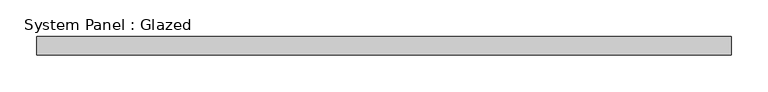
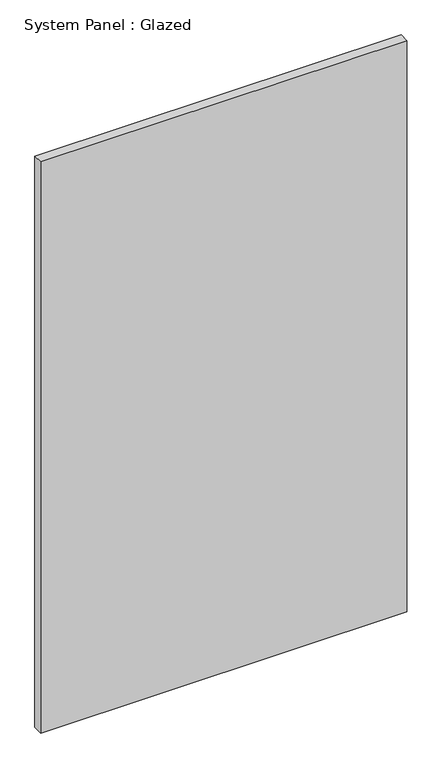
"""IFC4 building model written with IfcOpenShell, lengths in millimetres: plate geometry, System Panel : Glazed."""

from ifc_helpers import new_model, si_unit, origin, origin_with_axes, place, context, project, spatial, polyline, outline, extrude, source, transform, mapped, element, save


def system_panel_glazed_239ce734(model_context):
    return source(origin(), model_context, "Body", "SweptSolid", [
        extrude(outline(polyline([(473.075, 19.05), (-473.075, 19.05), (-473.075, 44.45), (473.075, 44.45), (473.075, 19.05)])), origin_with_axes(), (0.0, 0.0, 1.0), 1559.8910355),
    ])


if __name__ == "__main__":
    model = new_model("IFC4")
    model_context = context("Model", 3, world=origin())
    ifc_project = project(units=[si_unit("LENGTHUNIT", "METRE", prefix="MILLI")], contexts=[model_context])
    site = spatial("IfcSite", under=ifc_project)
    building = spatial("IfcBuilding", under=site)
    placement = place(None, origin())
    system_panel_glazed_shape = system_panel_glazed_239ce734(model_context)
    element("IfcPlate", 1, ObjectType="System Panel : Glazed", at=placement, inside=building, context=model_context, shape_type="MappedRepresentation", body=[
        mapped(system_panel_glazed_shape, transform((0.0, 0.0, 0.0), x_axis=(1.0, 0.0, 0.0), y_axis=(0.0, 1.0, 0.0), z_axis=(0.0, 0.0, 1.0))),
    ])
    save(model, "model.ifc")

# Revit data of these elements
# Type "System Panel : Glazed"
#   Construction Type Id = "GSP4R"
#   Analytic Construction = "1/8 in Pilkington single glazing"
#   Visual Light Transmittance = 0.9
#   Solar Heat Gain Coefficient = 0.86
#   Heat Transfer Coefficient (U) = 1.18115 BTU/(h·ft²·°F)
#   Define Thermal Properties by = 1
# Element 1 (IfcPlate, "System Panel : Glazed")
#   Materials on its faces: "Glass"
# Materials
#   "Glass": class "Glass", colour RGB 0 128 192, transparency 0.75, Description = "Soda Lime Glass", Cost = 0
